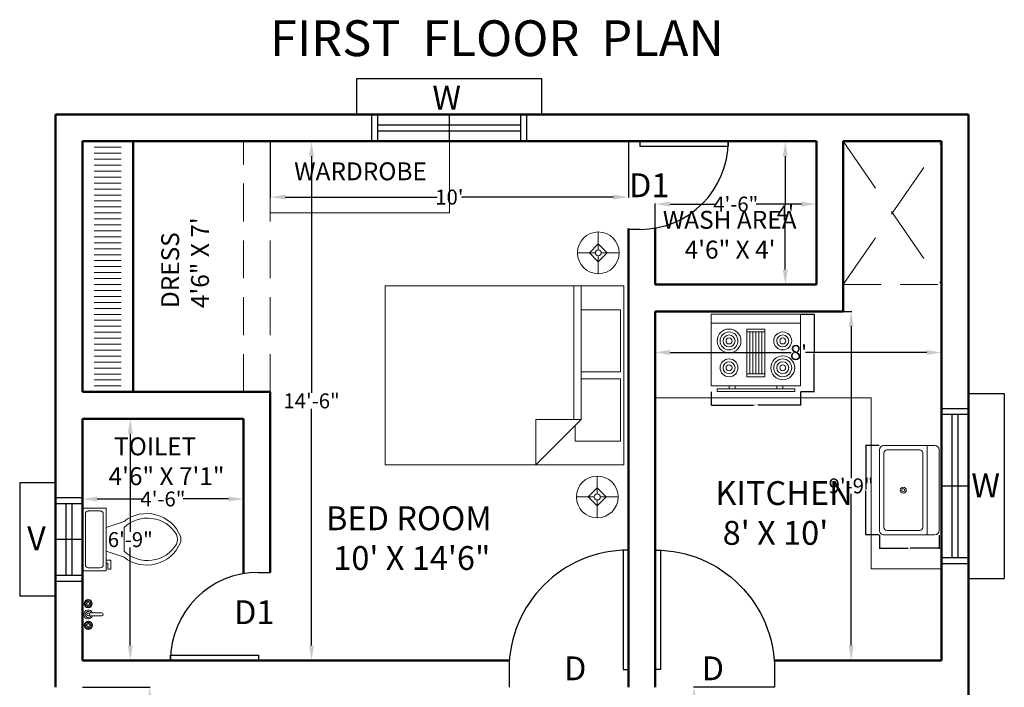
# Model space of a CAD drawing. Units: inches. Extents: x -25 to 789, y -921 to 230.
# Tile 5 of 5: x 437 to 767, y 6 to 230. Entities that reach past the tile are written whole.
import ezdxf

# ---------------------------------------------------------------- set-up
doc = ezdxf.new("R2010")
doc.units = ezdxf.units.IN
doc.header["$MEASUREMENT"] = 0
doc.linetypes.add('DASHED', pattern=[19.05, 12.7, -6.35])
for name, color, linetype, lineweight in [('A-ANNO-DIMS', 2, 'Continuous', 18), ('A-ANNO-TEXT', 7, 'Continuous', 18), ('A-AREA-IDEN', 3, 'Continuous', 18), ('A-DOOR', 4, 'Continuous', 25), ('A-FLOR-FIXT', 9, 'Continuous', 18), ('A-FLOR-OVHD', 8, 'DASHED', 18), ('A-FURN', 8, 'Continuous', 18), ('A-GLAZ', 4, 'Continuous', 25), ('A-WALL', 7, 'Continuous', 50), ('E-LITE-FIXT', 6, 'Continuous', 18)]:
    doc.layers.add(name, color=color, linetype=linetype, lineweight=lineweight)
doc.styles.get("Standard").update_dxf_attribs({"font": 'arial.ttf'})
doc.dimstyles.get("Standard").update_dxf_attribs({"dimtxt": 0.18, "dimasz": 0.18, "dimexe": 0.18, "dimexo": 0.0625, "dimgap": 0.09, "dimtad": 0, "dimtih": 1, "dimtoh": 1, "dimdec": 1, "dimzin": 0, "dimdsep": 46, "dimlunit": 4, "dimtxsty": 'Standard', "dimcen": 0.09, "dimadec": 0, "dimazin": 0, "dimtfac": 1, "dimtdec": 1, "dimtofl": 0, "dimtmove": 0, "dimatfit": 3, "dimfxl": 1, "dimtolj": 1, "dimtzin": 0, "dimarcsym": 0})

# ---------------------------------------------------------------- blocks, each defined once
blk = doc.blocks.new('*U20')
for p, q in [((-750, 0), (-750, 100)), ((0, 0), (0, 100))]:
    blk.add_line(p, q)
blk.add_lwpolyline([(0, 0), (0, -750), (-43.75, -750), (-43.75, 0)], close=True)
blk.add_arc((0, 0), 750, 180, 270)
blk = doc.blocks.new('Faucet - Bathroom top')
for p, q in [((-4.107, 0.125), (-4.375, 0.125)), ((-3.75, 0.4788), (-3.75, 0.75)), ((-3.5, 0.482), (-3.5, 0.75)), ((-3.1461, 0.125), (-2.875, 0.125)), ((3.143, 0.125), (2.875, 0.125)), ((3.5, 0.4788), (3.5, 0.75)), ((3.75, 0.482), (3.75, 0.75)), ((4.1039, 0.125), (4.375, 0.125)), ((-4.1039, -0.125), (-4.375, -0.125)), ((-3.75, -0.4821), (-3.75, -0.75)), ((-3.5, -0.4789), (-3.5, -0.75)), ((-3.143, -0.125), (-2.875, -0.125)), ((-0.5, -0.8639), (-0.5, -4.5)), ((0.5, -4.5), (0.5, -0.8631)), ((3.1461, -0.125), (2.875, -0.125)), ((3.5, -0.4821), (3.5, -0.75)), ((3.75, -0.4789), (3.75, -0.75)), ((4.107, -0.125), (4.375, -0.125))]:
    blk.add_line(p, q)
for centre, radius in [((-3.625, 0), 1.375), ((-4.625, 0), 0.2795), ((-3.625, 0), 0.5), ((-3.625, 1), 0.2795), ((-2.625, 0), 0.2795), ((0, 0), 0.5), ((3.625, 0), 1.375), ((2.625, 0), 0.2795), ((3.625, 0), 0.5), ((3.625, 1), 0.2795), ((4.625, 0), 0.2795), ((-3.625, -1), 0.2795), ((3.625, -1), 0.2795)]:
    blk.add_circle(centre, radius)
for centre, radius, start, end in [((-3.625, 0), 1, 105.2407, 164.2093), ((-3.625, 0), 1, 16.44125, 74.07887), ((0, 0), 1.5, 289.6514, 250.3603), ((0, 0), 1, 300.3431, 239.7554), ((3.625, 0), 1, 106.12, 164.0884), ((3.625, 0), 1, 16.23422, 73.90469), ((-3.625, 0), 1, 196.2342, 253.9047), ((-3.625, 0), 1, 286.12, 344.0884), ((3.625, 0), 1, 196.4413, 254.0789), ((3.625, 0), 1, 285.2407, 344.2093), ((0, -4.5), 0.5, 180, 0)]:
    blk.add_arc(centre, radius, start, end)
blk = doc.blocks.new('*U2')
for p, q in [((0, 0), (0, -6)), ((-40, 0), (-40, -6))]:
    blk.add_line(p, q)
blk.add_lwpolyline([(0, 0), (0, 40), (-1.75, 40), (-1.75, 0)], close=True)
blk.add_arc((0, 0), 40, 90, 180)
blk = doc.blocks.new('Bed - Queen')
for p, q in [((0, -80.00003), (0, 0)), ((0, 0), (59.99999, 0)), ((59.99999, 0), (59.99999, -80.00003)), ((7.99999, -1.2), (28.79998, -1.2)), ((7.99999, -14.4), (7.99999, -1.2)), ((28.79998, -1.2), (28.79998, -14.4)), ((31.19999, -1.2), (51.99999, -1.2)), ((31.19999, -14.4), (31.19999, -1.2)), ((51.99999, -1.2), (51.99999, -16.4)), ((0, -14.4), (44.8, -14.4)), ((59.99999, -29.6), (44.8, -14.4)), ((44.8, -14.4), (44.8, -29.6)), ((51.99999, -16.4), (46.79936, -16.4)), ((44.8, -16.8), (0, -16.8)), ((44.8, -29.6), (59.99999, -29.6)), ((59.99999, -80.00003), (0, -80.00003))]:
    blk.add_line(p, q)
blk = doc.blocks.new('Lamp - Table')
for p, q in [((0, 7), (0, 1)), ((-1, 0), (-7, 0)), ((0, 3), (-3, 0)), ((-3, 0), (0, -3)), ((3, 0), (0, 3)), ((0, -3), (3, 0)), ((1, 0), (7, 0)), ((0, -1), (0, -7))]:
    blk.add_line(p, q)
for radius in [7, 1]:
    blk.add_circle((0, 0), radius)
blk = doc.blocks.new('*U21')
for p, q in [((0, 0), (0, -100)), ((750, 0), (750, -100))]:
    blk.add_line(p, q)
blk.add_lwpolyline([(0, 0), (0, 750), (43.75, 750), (43.75, 0)], close=True)
blk.add_arc((0, 0), 750, 0, 90)
blk = doc.blocks.new('Range-Oven - 30 in top')
for p, q in [((0, -3), (30, -3)), ((12, -6), (18, -6)), ((13, -20), (13, -6)), ((14, -6), (14, -20)), ((15, -20), (15, -6)), ((16, -6), (16, -20)), ((17, -20), (17, -6)), ((18, -20), (12, -20)), ((6, -24), (6, -25)), ((8, -25), (8, -24)), ((22, -25), (22, -24)), ((24, -24), (24, -25))]:
    blk.add_line(p, q)
for points in [[(0, -24), (0, 0), (30, 0), (30, -24)], [(12, -21), (12, -5), (18, -5), (18, -21)], [(2, -26), (2, -25), (28, -25), (28, -26)]]:
    blk.add_lwpolyline(points, close=True)
for centre, radius in [((6, -9), 4), ((6, -9), 3), ((24, -9), 3), ((6, -9), 2), ((6, -9), 1), ((24, -9), 2), ((24, -9), 1), ((6, -18), 3), ((6, -18), 2), ((24, -18), 4), ((24, -18), 3), ((24, -18), 2), ((6, -18), 1), ((24, -18), 1)]:
    blk.add_circle(centre, radius)
blk = doc.blocks.new('Sink-single - 30 in top')
blk.add_line((-15, -3.999996), (15, -3.999996))
for points in [[(-13.5, 0), (13.5, 0)], [(-15, -18.499996), (-15, -1.5)], [(15, -1.5), (15, -18.499996)], [(-13.5, -17.499996), (-13.5, -6.499996)], [(-12.5, -5.499996), (12.5, -5.499996)], [(13.5, -6.499996), (13.5, -17.499996)], [(12.5, -18.499996), (-12.5, -18.499996)], [(13.5, -19.999996), (-13.5, -19.999996)]]:
    blk.add_lwpolyline(points)
for radius in [1, 0.5]:
    blk.add_circle((0, -11.999996), radius)
for centre, radius, start, end in [((-13.5, -1.5), 1.5, 90, 180), ((13.5, -1.5), 1.5, 0, 90), ((-12.5, -6.499996), 1, 90, 180), ((12.5, -6.499996), 1, 0, 90), ((-13.5, -18.499996), 1.5, 180, 270), ((-12.5, -17.499996), 1, 180, 270), ((12.5, -17.499996), 1, 270, 0), ((13.5, -18.499996), 1.5, 270, 0)]:
    blk.add_arc(centre, radius, start, end)
blk = doc.blocks.new('Toilet - top')
for p, q in [((9.5, -6), (9.5, -2)), ((-10, -8.5), (-8, -8.5)), ((-10, -9.5), (-10, -8.5)), ((-7, -9.5), (-10, -9.5)), ((-8, -8.5), (-8, -8)), ((-7, -8), (-7, -9.5)), ((-4, -8), (-6, -14)), ((4, -8), (6, -14)), ((4, -14), (-4, -14))]:
    blk.add_line(p, q)
blk.add_lwpolyline([(10.5, -8), (10.5, 0), (-10.5, 0), (-10.5, -8)], close=True)
for points in [[(-9.5, -2), (-9.5, -6)], [(8.5, -1), (-8.5, -1)], [(-8.5, -7), (8.5, -7)]]:
    blk.add_lwpolyline(points)
for centre, radius, start, end in [((-8.62, -1.88), 0.884, 81.8699, 188.1301), ((8.62, -1.88), 0.884, 351.8699, 98.1301), ((-8.62, -6.12), 0.884, 171.8699, 278.1301), ((8.62, -6.12), 0.884, 261.8699, 8.1301), ((3.52, -21.58), 12.17, 141.4691, 247.9714), ((4.2, -21.82), 11.33, 136.3677, 238.9468), ((-3.52, -21.58), 12.17, 292.0284, 38.5307), ((-4.2, -21.82), 11.33, 301.053, 43.6321), ((0, -27.88), 4, 245.7318, 294.2682), ((0, -29), 4, 254.8605, 285.1395)]:
    blk.add_arc(centre, radius, start, end)
blk = doc.blocks.new('*D61')
at = {"layer": 'A-ANNO-DIMS', "color": 0, "lineweight": -2, "transparency": 16777216}
for p, q in [((458.3, 6.3), (480.99, 6.3)), ((480.81, 1.3), (480.81, -15.11)), ((480.81, -36.7), (480.81, -20.29)), ((458.3, -41.7), (480.99, -41.7))]:
    blk.add_line(p, q, dxfattribs=at)
at = {"layer": 'A-ANNO-DIMS', "color": 0, "transparency": 16777216}
for points in [[(479.97, 1.3), (481.64, 1.3), (480.81, 6.3)], [(479.97, -36.7), (481.64, -36.7), (480.81, -41.7)]]:
    blk.add_solid(points, dxfattribs=at)
at = {"layer": 'Defpoints', "color": 0, "transparency": 16777216}
for p in [(458.24, 6.3), (480.81, 6.3), (458.24, -41.7)]:
    blk.add_point(p, dxfattribs=at)
at = {"layer": 'A-ANNO-DIMS', "color": 0, "transparency": 16777216, "insert": (480.81, -17.7), "char_height": 5, "attachment_point": 5}
blk.add_mtext("\\A1;4'", dxfattribs=at)
blk = doc.blocks.new('*D63')
at = {"layer": 'A-ANNO-DIMS', "color": 0, "lineweight": -2, "transparency": 16777216}
for p, q in [((458.3, 96.3), (474.48, 96.3)), ((474.3, 91.3), (474.3, 58.44)), ((474.3, 20.3), (474.3, 53.15)), ((458.3, 15.3), (474.48, 15.3))]:
    blk.add_line(p, q, dxfattribs=at)
at = {"layer": 'A-ANNO-DIMS', "color": 0, "transparency": 16777216}
for points in [[(473.47, 91.3), (475.13, 91.3), (474.3, 96.3)], [(473.47, 20.3), (475.13, 20.3), (474.3, 15.3)]]:
    blk.add_solid(points, dxfattribs=at)
at = {"layer": 'Defpoints', "color": 0, "transparency": 16777216}
for p in [(458.24, 96.3), (474.3, 96.3), (458.24, 15.3)]:
    blk.add_point(p, dxfattribs=at)
at = {"layer": 'A-ANNO-DIMS', "color": 0, "transparency": 16777216, "insert": (474.3, 55.8), "char_height": 5, "attachment_point": 5}
blk.add_mtext('\\A1;6\'-9"', dxfattribs=at)
blk = doc.blocks.new('*D64')
at = {"layer": 'A-ANNO-DIMS', "color": 0, "lineweight": -2, "transparency": 16777216}
for p, q in [((458.24, 96.23), (458.24, 69.24)), ((512.24, 96.23), (512.24, 69.24)), ((463.24, 69.42), (478.4, 69.42)), ((507.24, 69.42), (492.07, 69.42))]:
    blk.add_line(p, q, dxfattribs=at)
at = {"layer": 'A-ANNO-DIMS', "color": 0, "transparency": 16777216}
for points in [[(463.24, 70.25), (463.24, 68.58), (458.24, 69.42)], [(507.24, 70.25), (507.24, 68.58), (512.24, 69.42)]]:
    blk.add_solid(points, dxfattribs=at)
at = {"layer": 'Defpoints', "color": 0, "transparency": 16777216}
for p in [(458.24, 96.3), (512.24, 96.3), (512.24, 69.42)]:
    blk.add_point(p, dxfattribs=at)
at = {"layer": 'A-ANNO-DIMS', "color": 0, "transparency": 16777216, "insert": (485.24, 69.42), "char_height": 5, "attachment_point": 5}
blk.add_mtext('\\A1;4\'-6"', dxfattribs=at)
blk = doc.blocks.new('*D65')
at = {"layer": 'A-ANNO-DIMS', "color": 0, "lineweight": -2, "transparency": 16777216}
for p, q in [((521.24, 189.23), (521.24, 170.42)), ((641.24, 189.23), (641.24, 170.42)), ((526.24, 170.6), (577.14, 170.6)), ((636.24, 170.6), (585.33, 170.6))]:
    blk.add_line(p, q, dxfattribs=at)
at = {"layer": 'A-ANNO-DIMS', "color": 0, "transparency": 16777216}
for points in [[(526.24, 171.44), (526.24, 169.77), (521.24, 170.6)], [(636.24, 171.44), (636.24, 169.77), (641.24, 170.6)]]:
    blk.add_solid(points, dxfattribs=at)
at = {"layer": 'Defpoints', "color": 0, "transparency": 16777216}
for p in [(521.24, 189.3), (641.24, 189.3), (641.24, 170.6)]:
    blk.add_point(p, dxfattribs=at)
at = {"layer": 'A-ANNO-DIMS', "color": 0, "transparency": 16777216, "insert": (581.24, 170.6), "char_height": 5, "attachment_point": 5}
blk.add_mtext("\\A1;10'", dxfattribs=at)
blk = doc.blocks.new('*D66')
at = {"layer": 'A-ANNO-DIMS', "color": 0, "lineweight": -2, "transparency": 16777216}
for p, q in [((521.3, 189.3), (535.24, 189.3)), ((535.06, 184.3), (535.06, 104.94)), ((535.06, 20.3), (535.06, 99.65)), ((521.3, 15.3), (535.24, 15.3))]:
    blk.add_line(p, q, dxfattribs=at)
at = {"layer": 'A-ANNO-DIMS', "color": 0, "transparency": 16777216}
for points in [[(534.23, 184.3), (535.89, 184.3), (535.06, 189.3)], [(534.23, 20.3), (535.89, 20.3), (535.06, 15.3)]]:
    blk.add_solid(points, dxfattribs=at)
at = {"layer": 'Defpoints', "color": 0, "transparency": 16777216}
for p in [(521.24, 189.3), (521.24, 15.3), (535.06, 15.3)]:
    blk.add_point(p, dxfattribs=at)
at = {"layer": 'A-ANNO-DIMS', "color": 0, "transparency": 16777216, "insert": (535.06, 102.3), "char_height": 5, "attachment_point": 5}
blk.add_mtext('\\A1;14\'-6"', dxfattribs=at)
blk = doc.blocks.new('*D67')
at = {"layer": 'A-ANNO-DIMS', "color": 0, "lineweight": -2, "transparency": 16777216}
for p, q in [((650.24, 141.36), (650.24, 168.43)), ((704.24, 141.36), (704.24, 168.43)), ((655.24, 168.25), (670.4, 168.25)), ((699.24, 168.25), (684.07, 168.25))]:
    blk.add_line(p, q, dxfattribs=at)
at = {"layer": 'A-ANNO-DIMS', "color": 0, "transparency": 16777216}
for points in [[(655.24, 169.08), (655.24, 167.42), (650.24, 168.25)], [(699.24, 169.08), (699.24, 167.42), (704.24, 168.25)]]:
    blk.add_solid(points, dxfattribs=at)
at = {"layer": 'Defpoints', "color": 0, "transparency": 16777216}
for p in [(704.24, 168.25), (650.24, 141.3), (704.24, 141.3)]:
    blk.add_point(p, dxfattribs=at)
at = {"layer": 'A-ANNO-DIMS', "color": 0, "transparency": 16777216, "insert": (677.24, 168.25), "char_height": 5, "attachment_point": 5}
blk.add_mtext('\\A1;4\'-6"', dxfattribs=at)
blk = doc.blocks.new('*D68')
at = {"layer": 'A-ANNO-DIMS', "color": 0, "lineweight": -2, "transparency": 16777216}
for p, q in [((704.17, 189.3), (693.65, 189.3)), ((693.83, 184.3), (693.83, 167.89)), ((693.83, 146.3), (693.83, 162.71)), ((704.17, 141.3), (693.65, 141.3))]:
    blk.add_line(p, q, dxfattribs=at)
at = {"layer": 'A-ANNO-DIMS', "color": 0, "transparency": 16777216}
for points in [[(692.99, 184.3), (694.66, 184.3), (693.83, 189.3)], [(692.99, 146.3), (694.66, 146.3), (693.83, 141.3)]]:
    blk.add_solid(points, dxfattribs=at)
at = {"layer": 'Defpoints', "color": 0, "transparency": 16777216}
for p in [(693.83, 189.3), (704.24, 189.3), (704.24, 141.3)]:
    blk.add_point(p, dxfattribs=at)
at = {"layer": 'A-ANNO-DIMS', "color": 0, "transparency": 16777216, "insert": (693.83, 165.3), "char_height": 5, "attachment_point": 5}
blk.add_mtext("\\A1;4'", dxfattribs=at)
blk = doc.blocks.new('*D69')
at = {"layer": 'A-ANNO-DIMS', "color": 0, "lineweight": -2, "transparency": 16777216}
for p, q in [((650.24, 132.23), (650.24, 118.34)), ((746.24, 132.23), (746.24, 118.34)), ((655.24, 118.52), (695.84, 118.52)), ((741.24, 118.52), (700.63, 118.52))]:
    blk.add_line(p, q, dxfattribs=at)
at = {"layer": 'A-ANNO-DIMS', "color": 0, "transparency": 16777216}
for points in [[(655.24, 119.36), (655.24, 117.69), (650.24, 118.52)], [(741.24, 119.36), (741.24, 117.69), (746.24, 118.52)]]:
    blk.add_solid(points, dxfattribs=at)
at = {"layer": 'Defpoints', "color": 0, "transparency": 16777216}
for p in [(650.24, 132.3), (746.24, 132.3), (746.24, 118.52)]:
    blk.add_point(p, dxfattribs=at)
at = {"layer": 'A-ANNO-DIMS', "color": 0, "transparency": 16777216, "insert": (698.24, 118.52), "char_height": 5, "attachment_point": 5}
blk.add_mtext("\\A1;8'", dxfattribs=at)
blk = doc.blocks.new('*D70')
at = {"layer": 'A-ANNO-DIMS', "color": 0, "lineweight": -2, "transparency": 16777216}
for p, q in [((713.3, 132.3), (716.08, 132.3)), ((715.9, 127.3), (715.9, 76.44)), ((715.9, 20.3), (715.9, 71.15)), ((718.12, 15.3), (715.72, 15.3))]:
    blk.add_line(p, q, dxfattribs=at)
at = {"layer": 'A-ANNO-DIMS', "color": 0, "transparency": 16777216}
for points in [[(715.07, 127.3), (716.73, 127.3), (715.9, 132.3)], [(715.07, 20.3), (716.73, 20.3), (715.9, 15.3)]]:
    blk.add_solid(points, dxfattribs=at)
at = {"layer": 'Defpoints', "color": 0, "transparency": 16777216}
for p in [(713.24, 132.3), (715.9, 15.3), (718.18, 15.3)]:
    blk.add_point(p, dxfattribs=at)
at = {"layer": 'A-ANNO-DIMS', "color": 0, "transparency": 16777216, "insert": (715.9, 73.8), "char_height": 5, "attachment_point": 5}
blk.add_mtext('\\A1;9\'-9"', dxfattribs=at)
blk = doc.blocks.new('*D72')
at = {"layer": 'A-ANNO-DIMS', "color": 0, "lineweight": -2, "transparency": 16777216}
for p, q in [((690.17, 6.3), (663.04, 6.3)), ((663.22, 1.3), (663.22, -82.56)), ((663.22, -171.7), (663.22, -87.85)), ((670.23, -176.7), (663.04, -176.7))]:
    blk.add_line(p, q, dxfattribs=at)
at = {"layer": 'A-ANNO-DIMS', "color": 0, "transparency": 16777216}
for points in [[(662.38, 1.3), (664.05, 1.3), (663.22, 6.3)], [(662.38, -171.7), (664.05, -171.7), (663.22, -176.7)]]:
    blk.add_solid(points, dxfattribs=at)
at = {"layer": 'Defpoints', "color": 0, "transparency": 16777216}
for p in [(663.22, 6.3), (690.24, 6.3), (670.29, -176.7)]:
    blk.add_point(p, dxfattribs=at)
at = {"layer": 'A-ANNO-DIMS', "color": 0, "transparency": 16777216, "insert": (663.22, -85.2), "char_height": 5, "attachment_point": 5}
blk.add_mtext('\\A1;15\'-3"', dxfattribs=at)
blk = doc.blocks.new('WIN-W-SUNSHADE')
at = {"ltscale": 2}
for p, q in [((0, 9), (0, 21)), ((0, 21), (62, 21)), ((62, 9), (62, 21)), ((5, 9), (0, 9)), ((57, 9), (62, 9))]:
    blk.add_line(p, q, dxfattribs=at)
for p, q in [((5, 0), (5, 9)), ((57, 0), (57, 9))]:
    blk.add_line(p, q)
blk = doc.blocks.new('WIN-V-SUNSHADE')
for p, q in [((0, 9), (0, 21)), ((38, 21), (0, 21)), ((38, 9), (38, 21)), ((5, 9), (0, 9)), ((5, 0), (5, 9)), ((33, 0), (33, 9)), ((33, 9), (38, 9))]:
    blk.add_line(p, q)
blk = doc.blocks.new('*D101')
at = {"layer": 'A-ANNO-DIMS', "color": 0, "lineweight": -2, "transparency": 16777216}
for p, q in [((668.98, 105.33), (668.98, 100.71)), ((698.98, 105.33), (698.98, 100.71)), ((669.16, 100.89), (683.17, 100.89)), ((698.8, 100.89), (684.79, 100.89))]:
    blk.add_line(p, q, dxfattribs=at)
at = {"layer": 'A-ANNO-DIMS', "color": 0, "transparency": 16777216}
for points in [[(669.16, 100.92), (669.16, 100.86), (668.98, 100.89)], [(698.8, 100.92), (698.8, 100.86), (698.98, 100.89)]]:
    blk.add_solid(points, dxfattribs=at)
at = {"layer": 'Defpoints', "color": 0, "transparency": 16777216}
for p in [(668.98, 105.39), (698.98, 105.39), (698.98, 100.89)]:
    blk.add_point(p, dxfattribs=at)
at = {"layer": 'A-ANNO-DIMS', "color": 0, "transparency": 16777216, "insert": (683.98, 100.89), "char_height": 0.18, "attachment_point": 5}
blk.add_mtext('\\A1;RANGE 2\'-6"', dxfattribs=at)
blk = doc.blocks.new('*D102')
at = {"layer": 'A-ANNO-DIMS', "color": 0, "lineweight": -2, "transparency": 16777216}
for p, q in [((699.04, 131.39), (703.66, 131.39)), ((703.48, 131.21), (703.48, 118.57)), ((703.48, 105.57), (703.48, 118.21)), ((699.04, 105.39), (703.66, 105.39))]:
    blk.add_line(p, q, dxfattribs=at)
at = {"layer": 'A-ANNO-DIMS', "color": 0, "transparency": 16777216}
for points in [[(703.45, 131.21), (703.51, 131.21), (703.48, 131.39)], [(703.45, 105.57), (703.51, 105.57), (703.48, 105.39)]]:
    blk.add_solid(points, dxfattribs=at)
at = {"layer": 'Defpoints', "color": 0, "transparency": 16777216}
for p in [(698.98, 131.39), (703.48, 131.39), (698.98, 105.39)]:
    blk.add_point(p, dxfattribs=at)
at = {"layer": 'A-ANNO-DIMS', "color": 0, "transparency": 16777216, "insert": (703.48, 118.39), "char_height": 0.18, "attachment_point": 5}
blk.add_mtext('\\A1;2\'-2"', dxfattribs=at)
blk = doc.blocks.new('*D103')
at = {"layer": 'A-ANNO-DIMS', "color": 0, "lineweight": -2, "transparency": 16777216}
for p, q in [((725.32, 87.38), (720.7, 87.38)), ((720.88, 87.2), (720.88, 72.56)), ((720.88, 57.56), (720.88, 72.2)), ((725.32, 57.38), (720.7, 57.38))]:
    blk.add_line(p, q, dxfattribs=at)
at = {"layer": 'A-ANNO-DIMS', "color": 0, "transparency": 16777216}
for points in [[(720.85, 87.2), (720.91, 87.2), (720.88, 87.38)], [(720.85, 57.56), (720.91, 57.56), (720.88, 57.38)]]:
    blk.add_solid(points, dxfattribs=at)
at = {"layer": 'Defpoints', "color": 0, "transparency": 16777216}
for p in [(725.38, 87.38), (720.88, 57.38), (725.38, 57.38)]:
    blk.add_point(p, dxfattribs=at)
at = {"layer": 'A-ANNO-DIMS', "color": 0, "transparency": 16777216, "insert": (720.88, 72.38), "char_height": 0.18, "attachment_point": 5}
blk.add_mtext('\\A1;SINK 2\'-6"', dxfattribs=at)
blk = doc.blocks.new('*D104')
at = {"layer": 'A-ANNO-DIMS', "color": 0, "lineweight": -2, "transparency": 16777216}
for p, q in [((725.38, 57.32), (725.38, 52.7)), ((745.38, 57.32), (745.38, 52.7)), ((725.56, 52.88), (735.06, 52.88)), ((745.2, 52.88), (735.71, 52.88))]:
    blk.add_line(p, q, dxfattribs=at)
at = {"layer": 'A-ANNO-DIMS', "color": 0, "transparency": 16777216}
for points in [[(725.56, 52.91), (725.56, 52.85), (725.38, 52.88)], [(745.2, 52.91), (745.2, 52.85), (745.38, 52.88)]]:
    blk.add_solid(points, dxfattribs=at)
at = {"layer": 'Defpoints', "color": 0, "transparency": 16777216}
for p in [(725.38, 57.38), (745.38, 57.38), (745.38, 52.88)]:
    blk.add_point(p, dxfattribs=at)
at = {"layer": 'A-ANNO-DIMS', "color": 0, "transparency": 16777216, "insert": (735.38, 52.88), "char_height": 0.18, "attachment_point": 5}
blk.add_mtext('\\A1;1\'-8"', dxfattribs=at)

msp = doc.modelspace()

# ---------------------------------------------------------------- linework, layer by layer
at = {"layer": 'A-FLOR-OVHD'}
for p, q in [((512.24, 105.3), (512.24, 189.3)), ((521.24, 105.3), (521.24, 189.3)), ((713.24, 141.3), (746.24, 141.3))]:
    msp.add_line(p, q, dxfattribs=at)
at = {"layer": 'A-FLOR-OVHD', "ltscale": 1.5}
for p, q in [((713.24, 141.3), (746.24, 189.3)), ((713.24, 189.3), (746.24, 141.3))]:
    msp.add_line(p, q, dxfattribs=at)
at = {"layer": 'A-FURN'}
for p, q in [((521.24, 189.3), (521.24, 165.3)), ((581.24, 165.3), (581.24, 189.3)), ((462.24, 187.3), (471.24, 187.3)), ((462.24, 185.3), (471.24, 185.3)), ((462.24, 183.3), (471.24, 183.3)), ((462.24, 181.3), (471.24, 181.3)), ((462.24, 179.3), (471.24, 179.3)), ((462.24, 177.3), (471.24, 177.3)), ((462.24, 175.3), (471.24, 175.3)), ((462.24, 173.3), (471.24, 173.3)), ((462.24, 171.3), (471.24, 171.3)), ((462.24, 169.3), (471.24, 169.3)), ((462.24, 167.3), (471.24, 167.3)), ((462.24, 165.3), (471.24, 165.3)), ((521.24, 165.3), (581.24, 165.3)), ((462.24, 163.3), (471.24, 163.3)), ((462.24, 161.3), (471.24, 161.3)), ((462.24, 159.3), (471.24, 159.3)), ((462.24, 157.3), (471.24, 157.3)), ((462.24, 155.3), (471.24, 155.3)), ((462.24, 153.3), (471.24, 153.3)), ((462.24, 151.3), (471.24, 151.3)), ((462.24, 149.3), (471.24, 149.3)), ((462.24, 147.3), (471.24, 147.3)), ((462.24, 145.3), (471.24, 145.3)), ((462.24, 143.3), (471.24, 143.3)), ((462.24, 141.3), (471.24, 141.3)), ((462.24, 139.3), (471.24, 139.3)), ((462.24, 137.3), (471.24, 137.3)), ((462.24, 135.3), (471.24, 135.3)), ((462.24, 133.3), (471.24, 133.3)), ((704.24, 132.3), (650.24, 132.3)), ((462.24, 131.3), (471.24, 131.3)), ((462.24, 129.3), (471.24, 129.3)), ((462.24, 127.3), (471.24, 127.3)), ((462.24, 125.3), (471.24, 125.3)), ((462.24, 123.3), (471.24, 123.3)), ((462.24, 121.3), (471.24, 121.3)), ((462.24, 119.3), (471.24, 119.3)), ((462.24, 117.3), (471.24, 117.3)), ((462.24, 115.3), (471.24, 115.3)), ((462.24, 113.3), (471.24, 113.3)), ((462.24, 111.3), (471.24, 111.3)), ((462.24, 109.3), (471.24, 109.3)), ((462.24, 107.3), (471.24, 107.3)), ((650.24, 103.28), (722.62, 103.28)), ((722.62, 103.28), (722.62, 45.98)), ((722.62, 45.98), (746.24, 45.98))]:
    msp.add_line(p, q, dxfattribs=at)
at = {"layer": 'A-GLAZ'}
for p, q in [((557.24, 189.3), (557.24, 198.3)), ((581.24, 189.3), (581.24, 198.3)), ((605.24, 189.3), (605.24, 198.3)), ((557.24, 194.8), (605.24, 194.8)), ((557.24, 192.8), (605.24, 192.8)), ((746.24, 97.8), (755.24, 97.8)), ((749.74, 49.8), (749.74, 97.8)), ((751.74, 49.8), (751.74, 97.8)), ((746.24, 73.8), (755.24, 73.8)), ((458.24, 67.8), (449.24, 67.8)), ((452.74, 67.8), (452.74, 43.8)), ((454.74, 67.8), (454.74, 43.8)), ((458.24, 55.8), (449.24, 55.8)), ((746.24, 49.8), (755.24, 49.8)), ((458.24, 43.8), (449.24, 43.8))]:
    msp.add_line(p, q, dxfattribs=at)
at = {"layer": 'A-WALL'}
for p, q in [((449.24, 6.3), (449.24, 198.3)), ((449.24, 198.3), (521.24, 198.3)), ((521.24, 198.3), (650.24, 198.3)), ((650.24, 198.3), (755.24, 198.3)), ((755.24, 198.3), (755.24, 6.3)), ((458.24, 189.3), (521.24, 189.3)), ((458.24, 105.3), (458.24, 189.3)), ((458.24, 189.3), (475.24, 189.3)), ((475.24, 189.3), (475.24, 105.3)), ((521.24, 189.3), (641.24, 189.3)), ((641.24, 189.3), (704.24, 189.3)), ((704.24, 189.3), (704.24, 141.3)), ((713.24, 189.3), (713.24, 132.3)), ((713.24, 189.3), (746.24, 189.3)), ((746.24, 189.3), (746.24, 132.3)), ((641.24, 160.03), (641.24, 6.3)), ((650.24, 160.21), (650.24, 141.3)), ((704.24, 141.3), (650.24, 141.3)), ((650.24, 132.3), (713.24, 132.3)), ((650.24, 132.3), (650.24, 6.3)), ((746.24, 132.3), (746.24, 15.3)), ((521.24, 105.3), (458.24, 105.3)), ((521.24, 44.82), (521.24, 105.3)), ((512.24, 96.3), (458.24, 96.3)), ((458.24, 96.3), (458.24, 15.3)), ((512.24, 44.39), (512.24, 96.3)), ((521.24, 15.3), (458.24, 15.3)), ((601.35, 15.3), (521.24, 15.3)), ((746.24, 15.3), (690.12, 15.3)), ((755.24, 15.3), (755.24, -323.42))]:
    msp.add_line(p, q, dxfattribs=at)

# ---------------------------------------------------------------- block references
at = {"layer": 'A-DOOR', "xscale": 0.0393700787401575, "yscale": 0.0393700787401575, "zscale": 0.0393700787401575, "rotation": 270}
for name, p in [('*U21', (645.17, 189.3)), ('*U20', (517.3, 15.3))]:
    msp.add_blockref(name, p, dxfattribs=at)
at = {"layer": 'A-DOOR'}
msp.add_blockref('*U2', (641.24, 12.3), dxfattribs=at)
at = {"layer": 'A-DOOR', "xscale": -1}
msp.add_blockref('*U2', (650.24, 12.3), dxfattribs=at)
at = {"layer": 'A-FLOR-FIXT'}
msp.add_blockref('Range-Oven - 30 in top', (668.98, 131.39), dxfattribs=at)
for name, p, rotation in [('Sink-single - 30 in top', (745.38, 72.38), 270), ('Toilet - top', (458.24, 55.89), 90), ('Faucet - Bathroom top', (460.21, 30.71), 90.42077596570412)]:
    msp.add_blockref(name, p, dxfattribs=dict(at, rotation=rotation))
at = {"layer": 'A-FURN', "rotation": 270}
msp.add_blockref('Bed - Queen', (639.77, 140.84), dxfattribs=at)
at = {"layer": 'A-GLAZ'}
msp.add_blockref('WIN-W-SUNSHADE', (550.24, 189.3), dxfattribs=at)
for name, p, rotation in [('WIN-W-SUNSHADE', (746.24, 104.8), 270.0000000000002), ('WIN-V-SUNSHADE', (458.24, 36.8), 89.99999999999966)]:
    msp.add_blockref(name, p, dxfattribs=dict(at, rotation=rotation))
at = {"layer": 'E-LITE-FIXT'}
for p in [(631.17, 151.92), (630.81, 70.1)]:
    msp.add_blockref('Lamp - Table', p, dxfattribs=at)

# ---------------------------------------------------------------- texts
at = {"layer": 'A-ANNO-TEXT'}
for s, p in [('W', (575.55, 199.96)), ('D1', (641.45, 170.57)), ('W', (756.19, 69.97)), ('V', (439.72, 52.26)), ('D1', (509.07, 27.46)), ('D', (619.66, 8.65)), ('D', (665.78, 8.65))]:
    msp.add_text(s, height=8, dxfattribs=at).set_placement(p)
at = {"layer": 'A-ANNO-TEXT', "insert": (521.11, 229.85), "char_height": 12, "attachment_point": 1}
msp.add_mtext_dynamic_manual_height_columns('FIRST  FLOOR  PLAN', width=235.2118, gutter_width=1, heights=[0], dxfattribs=at)
at = {"layer": 'A-AREA-IDEN', "attachment_point": 1}
for s, insert, char_height in [('WARDROBE', (529.23, 182.24), 6), ('WASH AREA\\P    4\'6" X 4\'', (652.78, 165.99), 6), (' TOILET\\P4\'6" X 7\'1"', (467.03, 90.06), 6), ("KITCHEN\\P 8' X 10'", (670.4, 75.39), 8), ('BED ROOM\\P 10\' X 14\'6"', (539.89, 66.96), 8)]:
    msp.add_mtext_dynamic_manual_height_columns(s, width=99.8363, gutter_width=1, heights=[0], dxfattribs=dict(at, insert=insert, char_height=char_height))
at = {"layer": 'A-AREA-IDEN', "insert": (484.67, 133.4), "char_height": 6, "attachment_point": 1, "rotation": 90}
msp.add_mtext_dynamic_manual_height_columns('DRESS \\P4\'6" X 7\'', width=99.8363, gutter_width=1, heights=[0], dxfattribs=at)

# ---------------------------------------------------------------- dimensions: what is measured, and where the dimension line sits
at = {"layer": 'A-ANNO-DIMS'}
for base, p1, p2, override, picture, middle in [((641.24, 170.6), (521.24, 189.3), (641.24, 189.3), {"dimtxt": 5, "dimasz": 5, "dimclrd": 0, "dimclre": 0, "dimclrt": 0}, '*D65', (581.24, 170.6)), ((704.24, 168.25), (650.24, 141.3), (704.24, 141.3), {"dimtxt": 5, "dimasz": 5, "dimclrd": 0, "dimclre": 0, "dimclrt": 0}, '*D67', (677.24, 168.25)), ((746.24, 118.52), (650.24, 132.3), (746.24, 132.3), {"dimtxt": 5, "dimasz": 5, "dimclrd": 0, "dimclre": 0, "dimclrt": 0}, '*D69', (698.24, 118.52)), ((512.24, 69.42), (458.24, 96.3), (512.24, 96.3), {"dimtxt": 5, "dimasz": 5, "dimclrd": 0, "dimclre": 0, "dimclrt": 0}, '*D64', (485.24, 69.42)), ((745.38, 52.88), (725.38, 57.38), (745.38, 57.38), {"dimdec": 1, "dimrnd": 0, "dimzin": 1, "dimlunit": 4, "dimfrac": 2}, '*D104', (735.38, 52.88))]:
    dim = msp.add_linear_dim(base=base, p1=p1, p2=p2, dimstyle='Standard', override=override, dxfattribs=at)
    dim.commit()
    dim.dimension.update_dxf_attribs({"geometry": picture, "text_midpoint": middle})
for base, p1, p2, override, picture, middle in [((535.06, 15.3), (521.24, 189.3), (521.24, 15.3), {"dimtxt": 5, "dimasz": 5, "dimclrd": 0, "dimclre": 0, "dimclrt": 0}, '*D66', (535.06, 102.3)), ((693.83, 189.3), (704.24, 141.3), (704.24, 189.3), {"dimtxt": 5, "dimasz": 5, "dimclrd": 0, "dimclre": 0, "dimclrt": 0}, '*D68', (693.83, 165.3)), ((715.9, 15.3), (713.24, 132.3), (718.18, 15.3), {"dimtxt": 5, "dimasz": 5, "dimclrd": 0, "dimclre": 0, "dimclrt": 0}, '*D70', (715.9, 73.8)), ((703.48, 131.39), (698.98, 105.39), (698.98, 131.39), {"dimdec": 1, "dimrnd": 0, "dimzin": 1, "dimlunit": 4, "dimfrac": 2}, '*D102', (703.48, 118.39)), ((474.3, 96.3), (458.24, 15.3), (458.24, 96.3), {"dimtxt": 5, "dimasz": 5, "dimclrd": 0, "dimclre": 0, "dimclrt": 0}, '*D63', (474.3, 55.8)), ((480.81, 6.3), (458.24, -41.7), (458.24, 6.3), {"dimtxt": 5, "dimasz": 5, "dimclrd": 0, "dimclre": 0, "dimclrt": 0}, '*D61', (480.81, -17.7)), ((663.22, 6.3), (670.29, -176.7), (690.24, 6.3), {"dimtxt": 5, "dimasz": 5, "dimclrd": 0, "dimclre": 0, "dimclrt": 0}, '*D72', (663.22, -85.2))]:
    dim = msp.add_linear_dim(base=base, p1=p1, p2=p2, angle=90, dimstyle='Standard', override=override, dxfattribs=at)
    dim.commit()
    dim.dimension.update_dxf_attribs({"geometry": picture, "text_midpoint": middle})
dim = msp.add_linear_dim(base=(698.98, 100.89), p1=(668.98, 105.39), p2=(698.98, 105.39), text='RANGE <>', dimstyle='Standard', override={"dimdec": 1, "dimrnd": 0, "dimzin": 1, "dimlunit": 4, "dimfrac": 2}, dxfattribs=at)
dim.commit()
dim.dimension.update_dxf_attribs({"geometry": '*D101', "text_midpoint": (683.98, 100.89)})
dim = msp.add_linear_dim(base=(720.88, 57.38), p1=(725.38, 87.38), p2=(725.38, 57.38), angle=270, text='SINK <>', dimstyle='Standard', override={"dimdec": 1, "dimrnd": 0, "dimzin": 1, "dimlunit": 4, "dimfrac": 2}, dxfattribs=at)
dim.commit()
dim.dimension.update_dxf_attribs({"geometry": '*D103', "text_midpoint": (720.88, 72.38)})

doc.saveas('drawing.dxf')
